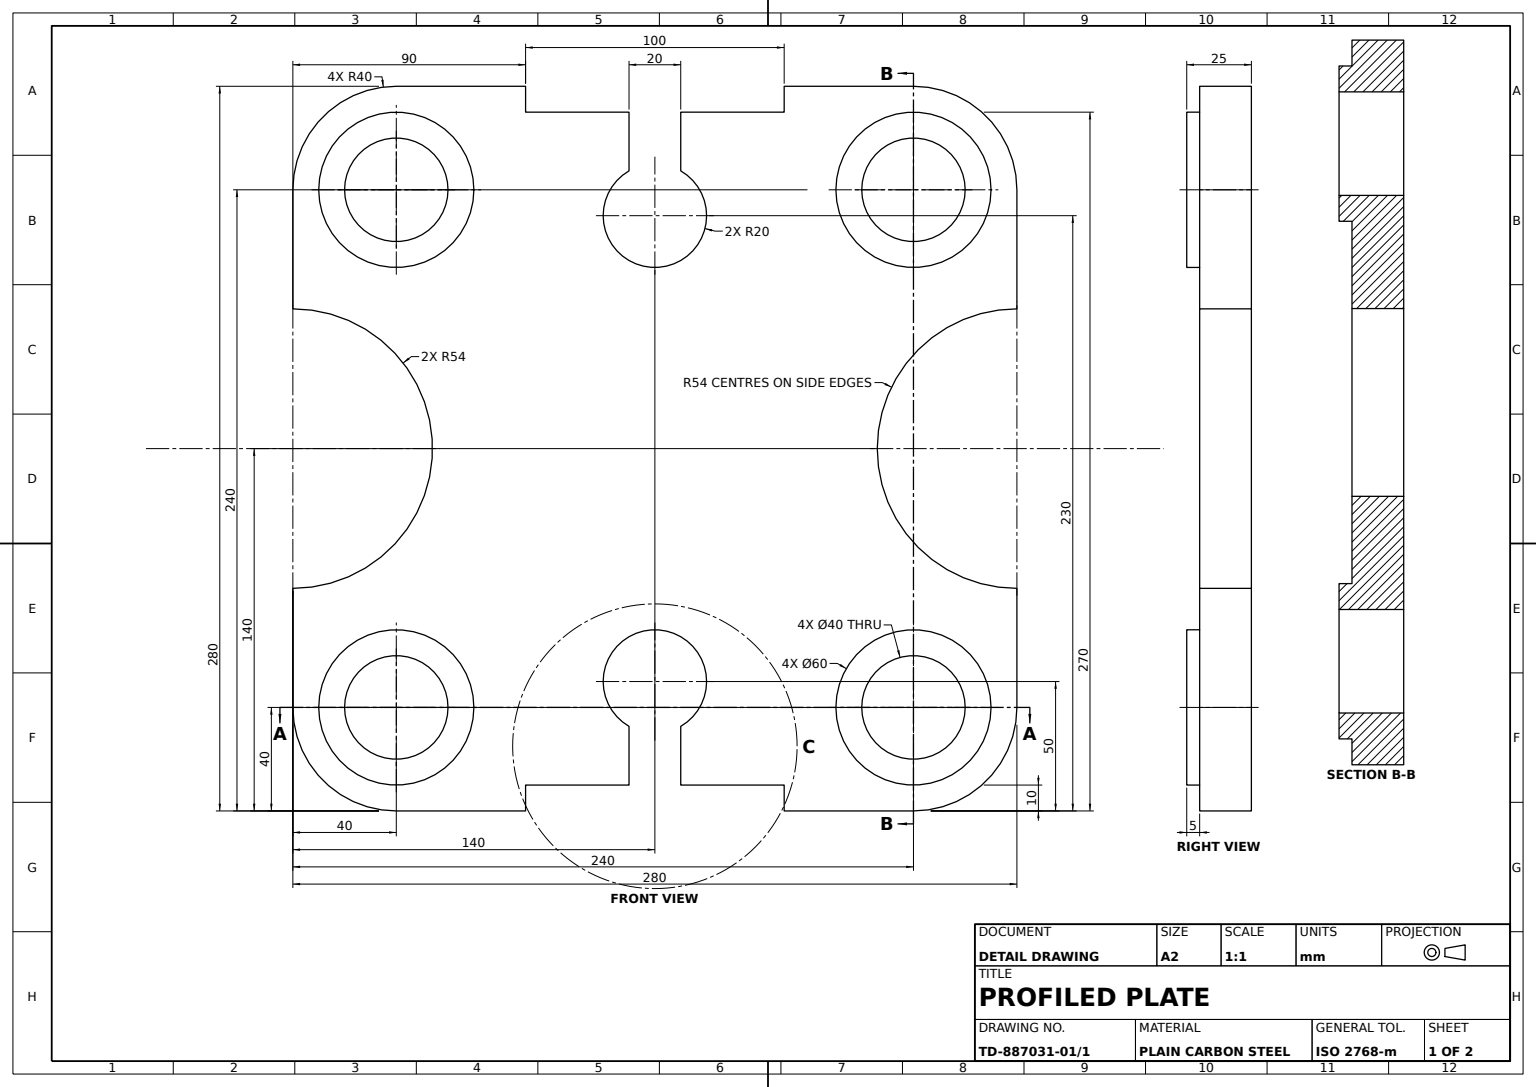
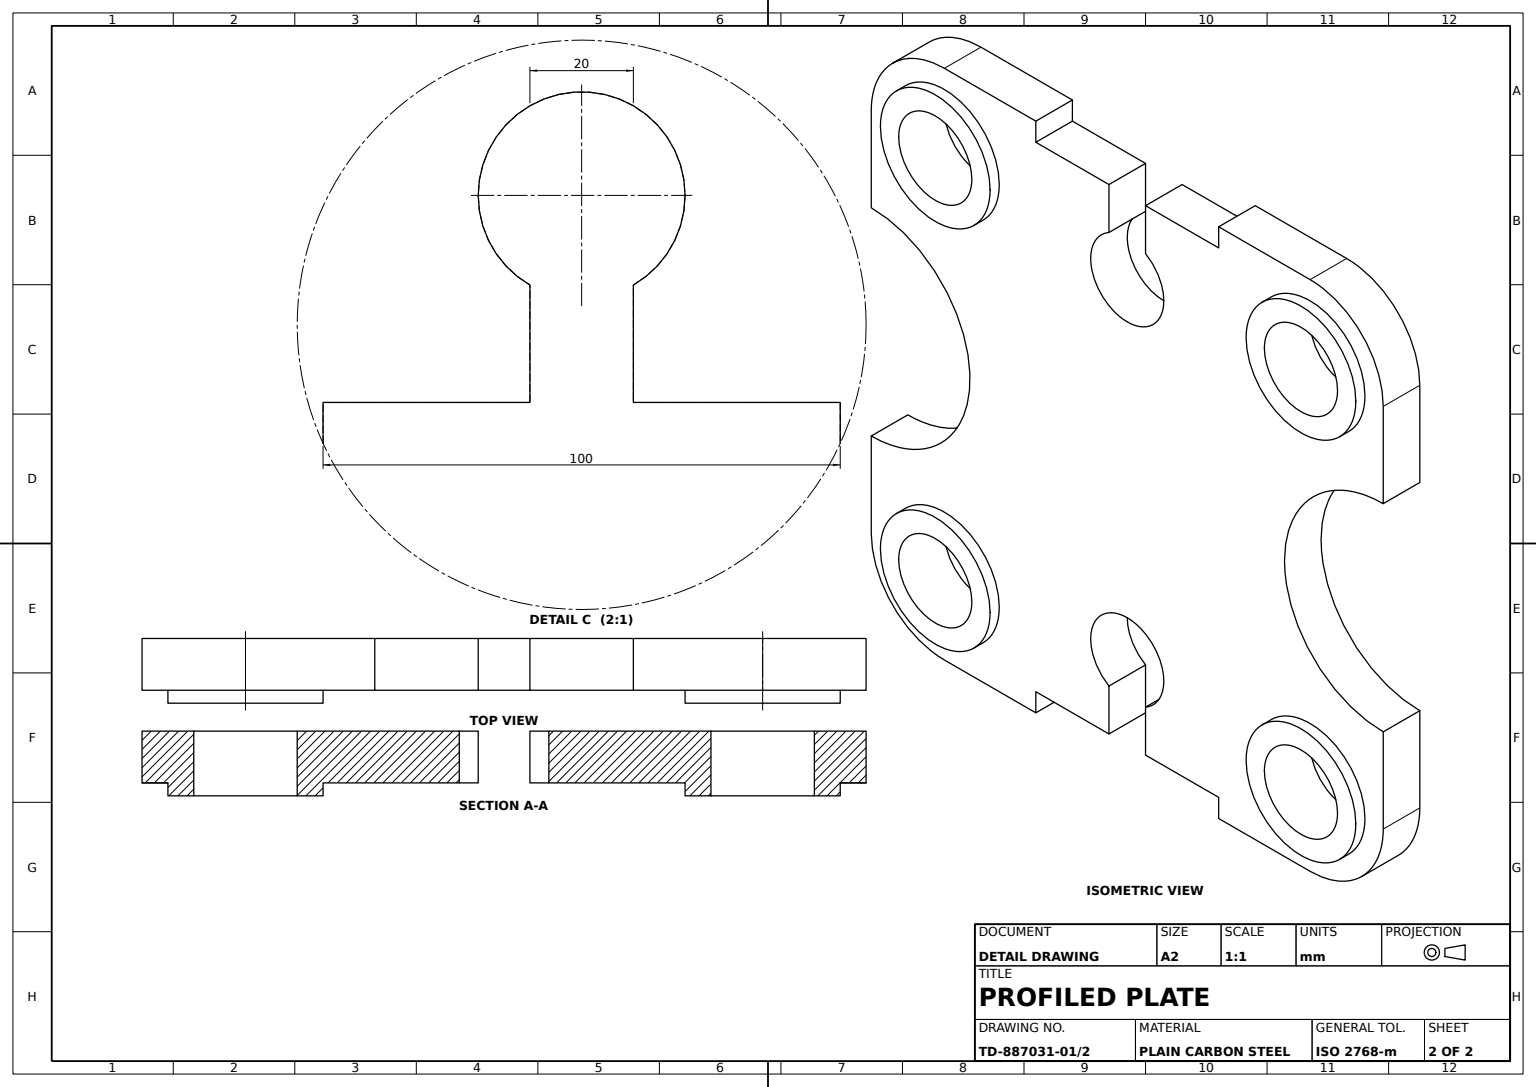
SolidWorks part; units mm, degrees
material "Plain Carbon Steel"
ref_plane "Front Plane" through (0, 0, 0) normal (0, 0, 1) x (1, 0, 0)
ref_plane "Top Plane" through (0, 0, 0) normal (0, 1, 0) x (1, 0, 0)
ref_plane "Right Plane" through (0, 0, 0) normal (1, 0, 0) x (0, 0, -1)
sketch "Plate Profile Sketch" plane through (0, 0, 0) normal (0, 0, 1) x (1, 0, 0)
  line L0 (40, 0) -> (90, 0)
  line L1 (90, 0) -> (90, 10)
  line L2 (90, 10) -> (130, 10)
  line L3 (190, 10) -> (190, 0)
  line L4 (190, 0) -> (240, 0)
  line L5 (280, 40) -> (280, 86)
  line L6 (240, 280) -> (190, 280)
  line L7 (190, 280) -> (190, 270)
  line L8 (190, 270) -> (150, 270)
  line L9 (90, 270) -> (90, 280)
  line L10 (90, 280) -> (40, 280)
  line L11 (0, 240) -> (0, 194)
  line L12 (0, 140) -> (280, 140) construction
  line L13 (140, 140) -> (140, 270) construction
  line L14 (140, 140) -> (140, 10) construction
  line L15 (140, 140) -> (140, 230) construction
  line L16 (140, 230) -> (170.3845, 230) construction
  line L17 (140, 230) -> (109.1584, 230) construction
  line L18 (0, 86) -> (0, 40)
  line L19 (280, 194) -> (280, 240)
  line L20 (140, 140) -> (140, 50) construction
  line L21 (130, 270) -> (130, 247.3205)
  line L23 (150, 270) -> (150, 247.3205)
  line L24 (130, 270) -> (90, 270)
  line L25 (130, 10) -> (130, 32.6795)
  line L27 (150, 10) -> (150, 32.6795)
  line L28 (150, 10) -> (190, 10)
  arc A0 (240, 280) -> (280, 240) centre (240, 240) cw
  arc A1 (280, 40) -> (240, 0) centre (240, 40) cw
  arc A2 (40, 0) -> (0, 40) centre (40, 40) cw
  arc A3 (0, 240) -> (40, 280) centre (40, 240) cw
  arc A4 (130, 247.3205) -> (150, 247.3205) centre (140, 230) ccw
  arc A5 (280, 194) -> (280, 86) centre (280, 140) ccw
  arc A6 (0, 86) -> (0, 194) centre (0, 140) ccw
  arc A7 (150, 32.6795) -> (130, 32.6795) centre (140, 50) ccw
  point P19 (0, 0)
  dimension "D1" = 40
  dimension "D2" = 40
  dimension "D3" = 50
  dimension "D9" = 108
  dimension "D10" = 108
  dimension "D21" = 40
  dimension "D4" = 100
  dimension "D5" = 10
  dimension "D6" = 50
  dimension "D7" = 100
  dimension "D8" = 50
  dimension "D11" = 100
  dimension "D12" = 240
  dimension "D13" = 86
  dimension "D14" = 240
  dimension "D15" = 270
  dimension "D16" = 240
  dimension "D17" = 20
  dimension "D18" = 10
  dimension "D19" = 230
  dimension "D20" = 247.3205
  dimension "D22" = 20
  dimension "D23" = 32.6795
  dimension "D24" = 140
  dimension "D25" = 50
extrude "Base Plate 20mm" add sketch "Plate Profile Sketch" along normal blind 20
sketch "Mounting Boss Rings Sketch" plane through (0, 0, 20) normal (0, 0, 1) x (1, 0, 0)
  circle A0 centre (240, 240) radius 20
  circle A1 centre (240, 240) radius 30
  circle A2 centre (40, 240) radius 30
  circle A3 centre (40, 240) radius 20
  circle A6 centre (240, 40) radius 20
  circle A7 centre (240, 40) radius 30
  circle A8 centre (40, 40) radius 20
  circle A9 centre (40, 40) radius 30
  dimension "D1" = 40
  dimension "D2" = 60
  dimension "D3" = 60
  dimension "D4" = 40
  dimension "D5" = 40
  dimension "D6" = 60
  dimension "D7" = 40
  dimension "D8" = 60
extrude "Mounting Bosses 4xØ60" add sketch "Mounting Boss Rings Sketch" along normal blind 5
sketch "Top Notch Sketch" plane through (0, 0, 20) normal (0, 0, 1) x (1, 0, 0)
  circle A0 centre (40, 240) radius 20
  circle A1 centre (240, 240) radius 20
  circle A2 centre (240, 40) radius 20
  circle A3 centre (40, 40) radius 20
  dimension "D1" = 40
extrude "Top Notch Cut" cut sketch "Top Notch Sketch" against normal through all
